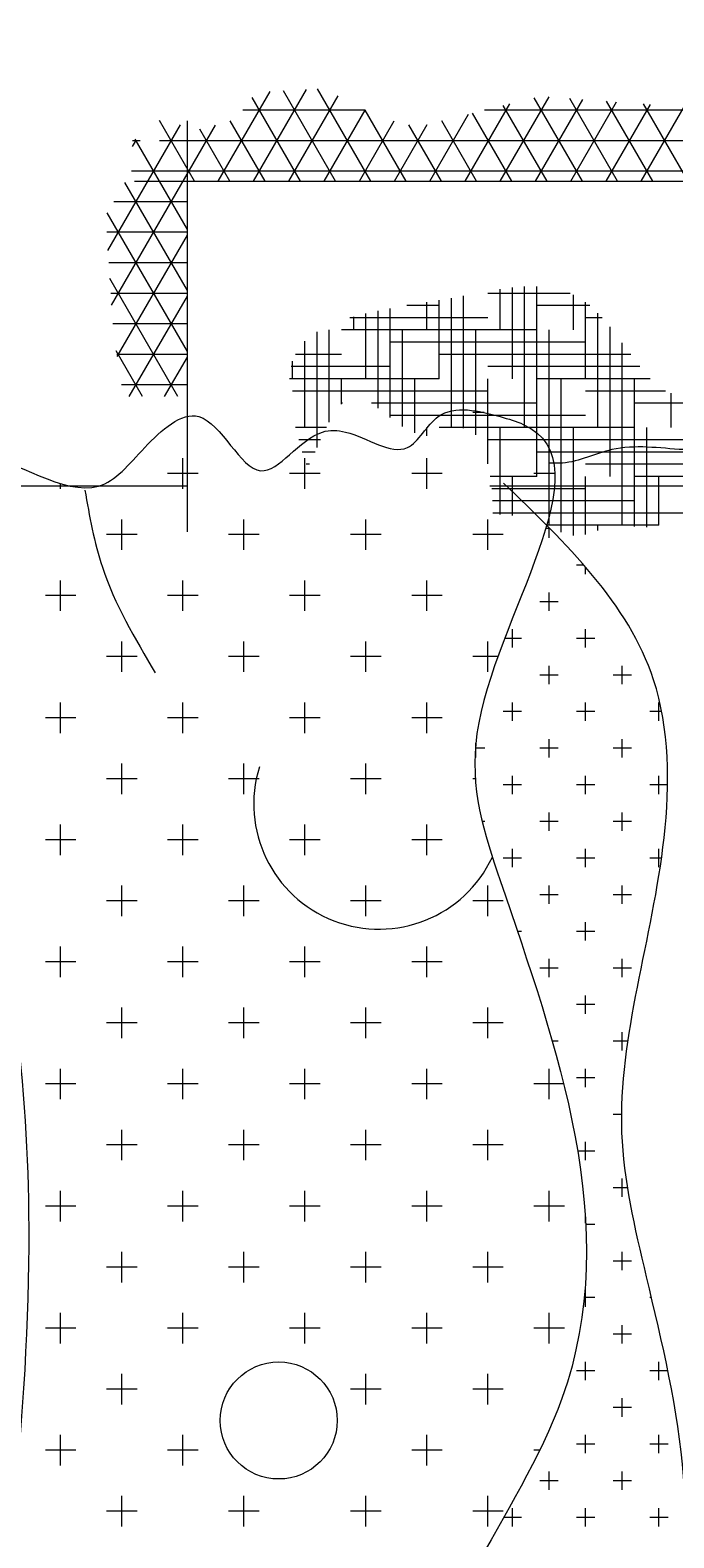
# Model space of a CAD drawing. Units: inches. Extents: x 3731 to 4318, y 1310 to 2388.
# Tile 5 of 57: x 3870 to 3897, y 1452 to 1515. Entities that reach past the tile are written whole.
import ezdxf

# ---------------------------------------------------------------- set-up
doc = ezdxf.new("R2010")
doc.units = ezdxf.units.IN
doc.layers.add('A-ANNO-DIMS', color=2, linetype='Continuous', lineweight=18)
doc.layers.add('A-FURN', color=8, linetype='Continuous', lineweight=13)
doc.styles.get("Standard").update_dxf_attribs({"font": 'arial.ttf'})
doc.dimstyles.get("Standard").update_dxf_attribs({"dimtxt": 0.18, "dimasz": 0.18, "dimexe": 0.18, "dimexo": 0.0625, "dimgap": 0.09, "dimtad": 0, "dimtih": 1, "dimtoh": 1, "dimdec": 4, "dimzin": 0, "dimdsep": 46, "dimtxsty": 'Standard', "dimcen": 0.09, "dimadec": 0, "dimazin": 0, "dimtfac": 1, "dimtdec": 4, "dimtofl": 0, "dimtmove": 0, "dimatfit": 3, "dimfxl": 1, "dimtolj": 1, "dimtzin": 0, "dimarcsym": 0})

# ---------------------------------------------------------------- blocks, each defined once
blk = doc.blocks.new('A$C200C7901')
for p, q in [((2, 1.6055), (2, 2.3334)), ((1.1379, 1.7195), (1.1379, 1.7508)), ((1.1222, 1.7352), (1.1535, 1.7352)), ((1.9972, 1.7352), (2.0027, 1.7352)), ((1.9972, 1.7352), (2.0027, 1.7352)), ((2, 1.6963), (2, 1.7248)), ((2, 1.6963), (2, 1.7248)), ((2.3121, 1.6596), (2.3121, 0.0201)), ((1.0129, 1.5945), (1.0129, 1.6258)), ((1.0129, 1.5945), (1.0129, 1.6258)), ((1.9533, 1.6055), (2.3741, 1.6055)), ((1.9533, 1.6055), (2.3741, 1.6055)), ((1.0754, 1.5625), (1.0754, 1.5633)), ((1.0754, 1.5625), (1.0754, 1.5633)), ((2, 0.2957), (2, 1.2957)), ((2.0224, 0.9977), (2.0224, 1.1977)), ((2.0224, 0.9977), (2.0224, 1.1977))]:
    blk.add_line(p, q)
at = {"linetype": 'ByBlock'}
for p, q in [((1.0129, 1.7195), (1.0129, 1.7508)), ((1.0129, 1.7195), (1.0129, 1.7508)), ((1.1379, 1.7195), (1.1379, 1.7508)), ((1.2629, 1.7195), (1.2629, 1.7508)), ((1.2629, 1.7195), (1.2629, 1.7508)), ((1.3879, 1.7195), (1.3879, 1.7508)), ((1.3879, 1.7195), (1.3879, 1.7508)), ((1.5129, 1.7195), (1.5129, 1.7508)), ((1.5129, 1.7195), (1.5129, 1.7508)), ((1.6379, 1.7195), (1.6379, 1.7508)), ((1.6379, 1.7195), (1.6379, 1.7508)), ((1.7629, 1.7195), (1.7629, 1.7508)), ((1.7629, 1.7195), (1.7629, 1.7508)), ((1.8879, 1.7195), (1.8879, 1.7508)), ((1.8879, 1.7195), (1.8879, 1.7508)), ((0.9972, 1.7352), (1.0285, 1.7352)), ((0.9972, 1.7352), (1.0285, 1.7352)), ((1.1222, 1.7352), (1.1535, 1.7352)), ((1.2472, 1.7352), (1.2785, 1.7352)), ((1.2472, 1.7352), (1.2785, 1.7352)), ((1.3722, 1.7352), (1.4035, 1.7352)), ((1.3722, 1.7352), (1.4035, 1.7352)), ((1.4972, 1.7352), (1.5285, 1.7352)), ((1.4972, 1.7352), (1.5285, 1.7352)), ((1.6222, 1.7352), (1.6535, 1.7352)), ((1.6222, 1.7352), (1.6535, 1.7352)), ((1.7472, 1.7352), (1.7785, 1.7352)), ((1.7472, 1.7352), (1.7785, 1.7352)), ((1.8722, 1.7352), (1.9035, 1.7352)), ((1.8722, 1.7352), (1.9035, 1.7352)), ((0.9504, 1.657), (0.9504, 1.6883)), ((0.9504, 1.657), (0.9504, 1.6883)), ((1.0754, 1.657), (1.0754, 1.6883)), ((1.0754, 1.657), (1.0754, 1.6883)), ((1.2004, 1.657), (1.2004, 1.6883)), ((1.2004, 1.657), (1.2004, 1.6883)), ((1.3254, 1.657), (1.3254, 1.6883)), ((1.3254, 1.657), (1.3254, 1.6883)), ((1.4504, 1.657), (1.4504, 1.6883)), ((1.4504, 1.657), (1.4504, 1.6883)), ((1.5754, 1.657), (1.5754, 1.6883)), ((1.5754, 1.657), (1.5754, 1.6883)), ((1.7004, 1.657), (1.7004, 1.6883)), ((1.7004, 1.657), (1.7004, 1.6883)), ((1.8254, 1.657), (1.8254, 1.6883)), ((1.8254, 1.657), (1.8254, 1.6883)), ((1.9504, 1.657), (1.9504, 1.6883)), ((1.9504, 1.657), (1.9504, 1.6883)), ((2.0919, 1.6152), (2.2125, 1.6848)), ((2.0919, 1.6152), (2.2125, 1.6848)), ((2.1377, 1.6055), (2.2798, 1.6876)), ((2.1377, 1.6055), (2.2798, 1.6876)), ((2.1854, 1.683), (2.3697, 1.5766)), ((2.1854, 1.683), (2.3697, 1.5766)), ((2.1974, 1.6055), (2.1974, 1.6838)), ((2.1974, 1.6055), (2.1974, 1.6838)), ((2.2287, 1.6055), (2.2287, 1.6859)), ((2.2287, 1.6055), (2.2287, 1.6859)), ((2.2414, 1.6868), (2.3699, 1.6126)), ((2.2414, 1.6868), (2.3699, 1.6126)), ((2.2599, 1.6055), (2.2599, 1.688)), ((2.2599, 1.6055), (2.2599, 1.688)), ((0.9347, 1.6727), (0.966, 1.6727)), ((0.9347, 1.6727), (0.966, 1.6727)), ((1.0597, 1.6727), (1.091, 1.6727)), ((1.0597, 1.6727), (1.091, 1.6727)), ((1.1847, 1.6727), (1.216, 1.6727)), ((1.1847, 1.6727), (1.216, 1.6727)), ((1.3097, 1.6727), (1.341, 1.6727)), ((1.3097, 1.6727), (1.341, 1.6727)), ((1.4347, 1.6727), (1.466, 1.6727)), ((1.4347, 1.6727), (1.466, 1.6727)), ((1.5597, 1.6727), (1.591, 1.6727)), ((1.5597, 1.6727), (1.591, 1.6727)), ((1.6847, 1.6727), (1.716, 1.6727)), ((1.6847, 1.6727), (1.716, 1.6727)), ((1.8097, 1.6727), (1.841, 1.6727)), ((1.8097, 1.6727), (1.841, 1.6727)), ((1.9347, 1.6727), (1.966, 1.6727)), ((1.9347, 1.6727), (1.966, 1.6727)), ((2.0919, 1.6513), (2.1386, 1.6782)), ((2.0919, 1.6513), (2.1386, 1.6782)), ((2.1037, 1.6055), (2.1037, 1.673)), ((2.1037, 1.6055), (2.1037, 1.673)), ((2.1327, 1.6773), (2.2571, 1.6055)), ((2.1327, 1.6773), (2.2571, 1.6055)), ((2.1349, 1.6055), (2.1349, 1.6777)), ((2.1349, 1.6055), (2.1349, 1.6777)), ((2.1662, 1.6055), (2.1662, 1.6817)), ((2.1662, 1.6055), (2.1662, 1.6817)), ((2.2002, 1.6055), (2.3109, 1.6694)), ((2.2002, 1.6055), (2.3109, 1.6694)), ((2.2912, 1.6055), (2.2912, 1.6809)), ((2.2912, 1.6055), (2.2912, 1.6809)), ((2.0919, 1.6649), (2.1946, 1.6055)), ((2.0919, 1.6649), (2.1946, 1.6055)), ((2.2627, 1.6055), (2.3551, 1.6589)), ((2.2627, 1.6055), (2.3551, 1.6589)), ((2.3224, 0.0468), (2.3224, 1.6627)), ((2.3224, 0.0468), (2.3224, 1.6627)), ((2.3476, 1.6616), (2.3547, 1.6575)), ((2.3476, 1.6616), (2.3547, 1.6575)), ((2.3537, 1.6539), (2.3537, 1.6616)), ((2.3537, 1.6539), (2.3537, 1.6616)), ((1.1379, 1.5945), (1.1379, 1.6258)), ((1.1379, 1.5945), (1.1379, 1.6258)), ((1.2629, 1.5945), (1.2629, 1.6258)), ((1.2629, 1.5945), (1.2629, 1.6258)), ((1.3879, 1.5945), (1.3879, 1.6258)), ((1.3879, 1.5945), (1.3879, 1.6258)), ((1.5129, 1.5945), (1.5129, 1.6258)), ((1.5129, 1.5945), (1.5129, 1.6258)), ((1.6379, 1.5945), (1.6379, 1.6258)), ((1.6379, 1.5945), (1.6379, 1.6258)), ((1.7629, 1.5945), (1.7629, 1.6258)), ((1.7629, 1.5945), (1.7629, 1.6258)), ((1.8879, 1.5945), (1.8879, 1.6258)), ((1.8879, 1.5945), (1.8879, 1.6258)), ((2.0129, 1.5945), (2.0129, 1.6258)), ((2.0129, 1.5945), (2.0129, 1.6258)), ((2.0919, 1.6288), (2.1321, 1.6055)), ((2.0919, 1.6288), (2.1321, 1.6055)), ((2.3121, 1.598), (2.3745, 1.634)), ((2.3121, 1.598), (2.3745, 1.634)), ((2.3537, 0.0056), (2.3537, 1.634)), ((2.3537, 0.0056), (2.3537, 1.634)), ((0.9972, 1.6102), (1.0285, 1.6102)), ((0.9972, 1.6102), (1.0285, 1.6102)), ((1.1222, 1.6102), (1.1535, 1.6102)), ((1.1222, 1.6102), (1.1535, 1.6102)), ((1.2472, 1.6102), (1.2785, 1.6102)), ((1.2472, 1.6102), (1.2785, 1.6102)), ((1.3722, 1.6102), (1.4035, 1.6102)), ((1.3722, 1.6102), (1.4035, 1.6102)), ((1.4972, 1.6102), (1.5285, 1.6102)), ((1.4972, 1.6102), (1.5285, 1.6102)), ((1.6222, 1.6102), (1.6535, 1.6102)), ((1.6222, 1.6102), (1.6535, 1.6102)), ((1.7472, 1.6102), (1.7785, 1.6102)), ((1.7472, 1.6102), (1.7785, 1.6102)), ((1.8722, 1.6102), (1.9035, 1.6102)), ((1.8722, 1.6102), (1.9035, 1.6102)), ((1.9972, 1.6102), (2.0285, 1.6102)), ((1.9972, 1.6102), (2.0285, 1.6102)), ((2.3121, 1.5619), (2.3654, 1.5926)), ((2.3121, 1.5619), (2.3654, 1.5926)), ((0.9504, 1.532), (0.9504, 1.5633)), ((0.9504, 1.532), (0.9504, 1.5633)), ((1.2004, 1.532), (1.2004, 1.5633)), ((1.2004, 1.532), (1.2004, 1.5633)), ((1.3254, 1.532), (1.3254, 1.5633)), ((1.3254, 1.532), (1.3254, 1.5633)), ((1.4504, 1.532), (1.4504, 1.5633)), ((1.4504, 1.532), (1.4504, 1.5633)), ((1.5754, 1.532), (1.5754, 1.5633)), ((1.5754, 1.532), (1.5754, 1.5633)), ((1.7004, 1.532), (1.7004, 1.5633)), ((1.7004, 1.532), (1.7004, 1.5633)), ((1.8254, 1.532), (1.8254, 1.5633)), ((1.8254, 1.532), (1.8254, 1.5633)), ((1.9504, 1.532), (1.9504, 1.5633)), ((1.9504, 1.532), (1.9504, 1.5633)), ((2.3121, 1.5738), (2.404, 1.5208)), ((2.3121, 1.5738), (2.404, 1.5208)), ((2.3121, 1.5258), (2.3739, 1.5615)), ((2.3121, 1.5258), (2.3739, 1.5615)), ((0.9347, 1.5477), (0.966, 1.5477)), ((0.9347, 1.5477), (0.966, 1.5477)), ((1.1847, 1.5477), (1.216, 1.5477)), ((1.1847, 1.5477), (1.216, 1.5477)), ((1.3097, 1.5477), (1.341, 1.5477)), ((1.3097, 1.5477), (1.341, 1.5477)), ((1.4347, 1.5477), (1.466, 1.5477)), ((1.4347, 1.5477), (1.466, 1.5477)), ((1.5597, 1.5477), (1.591, 1.5477)), ((1.5597, 1.5477), (1.591, 1.5477)), ((1.6847, 1.5477), (1.716, 1.5477)), ((1.6847, 1.5477), (1.716, 1.5477)), ((1.8097, 1.5477), (1.841, 1.5477)), ((1.8097, 1.5477), (1.841, 1.5477)), ((1.9347, 1.5477), (1.966, 1.5477)), ((1.9347, 1.5477), (1.966, 1.5477)), ((2.3849, 1.4236), (2.3849, 1.5486)), ((2.3849, 1.4236), (2.3849, 1.5486)), ((2.3121, 1.4897), (2.3979, 1.5393)), ((2.3121, 1.4897), (2.3979, 1.5393)), ((2.3121, 1.5377), (2.406, 1.4835)), ((2.3121, 1.5377), (2.406, 1.4835)), ((1.1379, 1.4695), (1.1379, 1.5008)), ((1.1379, 1.4695), (1.1379, 1.5008)), ((1.2629, 1.4695), (1.2629, 1.5008)), ((1.2629, 1.4695), (1.2629, 1.5008)), ((1.3879, 1.4695), (1.3879, 1.5008)), ((1.3879, 1.4695), (1.3879, 1.5008)), ((1.5129, 1.4695), (1.5129, 1.5008)), ((1.5129, 1.4695), (1.5129, 1.5008)), ((1.6379, 1.4695), (1.6379, 1.5008)), ((1.6379, 1.4695), (1.6379, 1.5008)), ((1.7629, 1.4695), (1.7629, 1.5008)), ((1.7629, 1.4695), (1.7629, 1.5008)), ((1.8879, 1.4695), (1.8879, 1.5008)), ((1.8879, 1.4695), (1.8879, 1.5008)), ((2.0129, 1.4695), (2.0129, 1.5008)), ((2.0129, 1.4695), (2.0129, 1.5008)), ((2.0974, 1.2977), (2.0974, 1.4977)), ((2.0974, 1.2977), (2.0974, 1.4977)), ((2.1099, 1.3477), (2.1099, 1.5009)), ((2.1099, 1.3477), (2.1099, 1.5009)), ((2.1099, 1.4977), (2.1279, 1.4977)), ((2.1099, 1.4977), (2.1279, 1.4977)), ((2.1224, 1.3977), (2.1224, 1.4992)), ((2.1224, 1.3977), (2.1224, 1.4992)), ((2.3121, 1.4537), (2.4047, 1.5071)), ((2.3121, 1.4537), (2.4047, 1.5071)), ((2.3121, 1.5016), (2.3997, 1.4511)), ((2.3121, 1.5016), (2.3997, 1.4511)), ((1.1222, 1.4852), (1.1535, 1.4852)), ((1.1222, 1.4852), (1.1535, 1.4852)), ((1.2472, 1.4852), (1.2785, 1.4852)), ((1.2472, 1.4852), (1.2785, 1.4852)), ((1.3722, 1.4852), (1.4035, 1.4852)), ((1.3722, 1.4852), (1.4035, 1.4852)), ((1.4972, 1.4852), (1.5285, 1.4852)), ((1.4972, 1.4852), (1.5285, 1.4852)), ((1.6222, 1.4852), (1.6535, 1.4852)), ((1.6222, 1.4852), (1.6535, 1.4852)), ((1.7472, 1.4852), (1.7785, 1.4852)), ((1.7472, 1.4852), (1.7785, 1.4852)), ((1.8722, 1.4852), (1.9035, 1.4852)), ((1.8722, 1.4852), (1.9035, 1.4852)), ((1.9972, 1.4852), (2.0285, 1.4852)), ((1.9972, 1.4852), (2.0285, 1.4852)), ((2.0224, 1.4805), (2.0224, 1.4839)), ((2.0224, 1.4805), (2.0224, 1.4839)), ((2.0349, 1.4748), (2.0349, 1.4879)), ((2.0349, 1.4748), (2.0349, 1.4879)), ((2.0474, 1.4691), (2.0474, 1.4915)), ((2.0474, 1.4691), (2.0474, 1.4915)), ((2.0599, 1.4631), (2.0599, 1.4948)), ((2.0599, 1.4631), (2.0599, 1.4948)), ((2.0599, 1.4852), (2.1484, 1.4852)), ((2.0599, 1.4852), (2.1484, 1.4852)), ((2.1349, 1.4477), (2.1349, 1.4949)), ((2.1349, 1.4477), (2.1349, 1.4949)), ((2.0397, 1.4727), (2.1581, 1.4727)), ((2.0397, 1.4727), (2.1581, 1.4727)), ((2.3121, 1.4176), (2.4067, 1.4721)), ((2.3121, 1.4176), (2.4067, 1.4721)), ((2.0656, 1.4602), (2.1599, 1.4602)), ((2.0656, 1.4602), (2.1599, 1.4602)), ((2.3121, 1.4655), (2.3849, 1.4235)), ((2.3121, 1.4655), (2.3849, 1.4235)), ((0.9504, 1.407), (0.9504, 1.4383)), ((0.9504, 1.407), (0.9504, 1.4383)), ((1.0754, 1.407), (1.0754, 1.4383)), ((1.0754, 1.407), (1.0754, 1.4383)), ((1.2004, 1.407), (1.2004, 1.4383)), ((1.2004, 1.407), (1.2004, 1.4383)), ((1.3254, 1.407), (1.3254, 1.4383)), ((1.3254, 1.407), (1.3254, 1.4383)), ((1.4504, 1.407), (1.4504, 1.4383)), ((1.4504, 1.407), (1.4504, 1.4383)), ((1.5754, 1.407), (1.5754, 1.4383)), ((1.5754, 1.407), (1.5754, 1.4383)), ((1.7004, 1.407), (1.7004, 1.4383)), ((1.7004, 1.407), (1.7004, 1.4383)), ((1.8254, 1.407), (1.8254, 1.4383)), ((1.8254, 1.407), (1.8254, 1.4383)), ((1.9504, 1.407), (1.9504, 1.4383)), ((1.9504, 1.407), (1.9504, 1.4383)), ((2.084, 1.4477), (2.1099, 1.4477)), ((2.084, 1.4477), (2.1099, 1.4477)), ((2.0849, 1.4468), (2.0849, 1.4477)), ((2.0849, 1.4468), (2.0849, 1.4477)), ((2.1599, 1.2477), (2.1599, 1.4477)), ((2.1599, 1.2477), (2.1599, 1.4477)), ((2.1724, 1.2977), (2.1724, 1.439)), ((2.1724, 1.2977), (2.1724, 1.439)), ((0.9347, 1.4227), (0.966, 1.4227)), ((0.9347, 1.4227), (0.966, 1.4227)), ((1.0597, 1.4227), (1.091, 1.4227)), ((1.0597, 1.4227), (1.091, 1.4227)), ((1.1847, 1.4227), (1.216, 1.4227)), ((1.1847, 1.4227), (1.216, 1.4227)), ((1.3097, 1.4227), (1.341, 1.4227)), ((1.3097, 1.4227), (1.341, 1.4227)), ((1.4347, 1.4227), (1.466, 1.4227)), ((1.4347, 1.4227), (1.466, 1.4227)), ((1.5597, 1.4227), (1.591, 1.4227)), ((1.5597, 1.4227), (1.591, 1.4227)), ((1.6847, 1.4227), (1.716, 1.4227)), ((1.6847, 1.4227), (1.716, 1.4227)), ((1.8097, 1.4227), (1.841, 1.4227)), ((1.8097, 1.4227), (1.841, 1.4227)), ((1.9347, 1.4227), (1.966, 1.4227)), ((1.9347, 1.4227), (1.966, 1.4227)), ((2.1099, 1.4227), (2.1767, 1.4227)), ((2.1099, 1.4227), (2.1767, 1.4227)), ((2.1599, 1.4352), (2.1735, 1.4352)), ((2.1599, 1.4352), (2.1735, 1.4352)), ((2.3121, 1.4294), (2.3741, 1.3937)), ((2.3121, 1.4294), (2.3741, 1.3937)), ((2.3121, 1.3815), (2.3848, 1.4235)), ((2.3121, 1.3815), (2.3848, 1.4235)), ((2.08, 1.4102), (2.1795, 1.4102)), ((2.08, 1.4102), (2.1795, 1.4102)), ((2.0849, 1.2477), (2.0849, 1.4171)), ((2.0849, 1.2477), (2.0849, 1.4171)), ((2.0703, 1.3977), (2.1819, 1.3977)), ((2.0703, 1.3977), (2.1819, 1.3977)), ((2.0724, 1.1977), (2.0724, 1.3977)), ((2.0724, 1.1977), (2.0724, 1.3977)), ((2.1474, 1.1977), (2.1474, 1.3977)), ((2.1474, 1.1977), (2.1474, 1.3977)), ((2.3121, 1.3934), (2.3703, 1.3598)), ((2.3121, 1.3934), (2.3703, 1.3598)), ((1.0129, 1.3445), (1.0129, 1.3758)), ((1.0129, 1.3445), (1.0129, 1.3758)), ((1.1379, 1.3445), (1.1379, 1.3758)), ((1.1379, 1.3445), (1.1379, 1.3758)), ((1.2629, 1.3445), (1.2629, 1.3758)), ((1.2629, 1.3445), (1.2629, 1.3758)), ((1.3879, 1.3445), (1.3879, 1.3758)), ((1.3879, 1.3445), (1.3879, 1.3758)), ((1.5129, 1.3445), (1.5129, 1.3758)), ((1.5129, 1.3445), (1.5129, 1.3758)), ((1.6379, 1.3445), (1.6379, 1.3758)), ((1.6379, 1.3445), (1.6379, 1.3758)), ((1.7629, 1.3445), (1.7629, 1.3758)), ((1.7629, 1.3445), (1.7629, 1.3758)), ((1.8879, 1.3445), (1.8879, 1.3758)), ((1.8879, 1.3445), (1.8879, 1.3758)), ((2.0129, 1.3445), (2.0129, 1.3758)), ((2.0129, 1.3445), (2.0129, 1.3758)), ((2.0612, 1.3852), (2.1599, 1.3852)), ((2.0612, 1.3852), (2.1599, 1.3852)), ((2.1849, 1.3477), (2.1849, 1.3808)), ((2.1849, 1.3477), (2.1849, 1.3808)), ((2.3121, 1.3454), (2.37, 1.3788)), ((2.3121, 1.3454), (2.37, 1.3788)), ((0.9972, 1.3602), (1.0285, 1.3602)), ((0.9972, 1.3602), (1.0285, 1.3602)), ((1.1222, 1.3602), (1.1535, 1.3602)), ((1.1222, 1.3602), (1.1535, 1.3602)), ((1.2472, 1.3602), (1.2785, 1.3602)), ((1.2472, 1.3602), (1.2785, 1.3602)), ((1.3722, 1.3602), (1.4035, 1.3602)), ((1.3722, 1.3602), (1.4035, 1.3602)), ((1.4972, 1.3602), (1.5285, 1.3602)), ((1.4972, 1.3602), (1.5285, 1.3602)), ((1.6222, 1.3602), (1.6535, 1.3602)), ((1.6222, 1.3602), (1.6535, 1.3602)), ((1.7472, 1.3602), (1.7785, 1.3602)), ((1.7472, 1.3602), (1.7785, 1.3602)), ((1.8722, 1.3602), (1.9035, 1.3602)), ((1.8722, 1.3602), (1.9035, 1.3602)), ((1.9972, 1.3602), (2.0285, 1.3602)), ((1.9972, 1.3602), (2.0285, 1.3602)), ((2.0515, 1.3602), (2.0599, 1.3602)), ((2.0515, 1.3602), (2.0599, 1.3602)), ((2.0545, 1.3727), (2.1099, 1.3727)), ((2.0545, 1.3727), (2.1099, 1.3727)), ((2.1599, 1.3602), (2.1883, 1.3602)), ((2.1599, 1.3602), (2.1883, 1.3602)), ((2.0599, 1.1477), (2.0599, 1.3477)), ((2.0599, 1.1477), (2.0599, 1.3477)), ((2.1099, 1.3477), (2.1904, 1.3477)), ((2.1099, 1.3477), (2.1904, 1.3477)), ((2.1349, 1.1515), (2.1349, 1.3477)), ((2.1349, 1.1515), (2.1349, 1.3477)), ((2.3121, 1.3573), (2.3808, 1.3176)), ((2.3121, 1.3573), (2.3808, 1.3176)), ((2.3121, 1.3093), (2.374, 1.345)), ((2.3121, 1.3093), (2.374, 1.345)), ((2.0599, 1.3352), (2.1926, 1.3352)), ((2.0599, 1.3352), (2.1926, 1.3352)), ((0.9504, 1.282), (0.9504, 1.3133)), ((0.9504, 1.282), (0.9504, 1.3133)), ((1.0754, 1.282), (1.0754, 1.3133)), ((1.0754, 1.282), (1.0754, 1.3133)), ((1.2004, 1.282), (1.2004, 1.3133)), ((1.2004, 1.282), (1.2004, 1.3133)), ((1.3254, 1.282), (1.3254, 1.3133)), ((1.3254, 1.282), (1.3254, 1.3133)), ((1.4504, 1.282), (1.4504, 1.3133)), ((1.4504, 1.282), (1.4504, 1.3133)), ((1.5754, 1.282), (1.5754, 1.3133)), ((1.5754, 1.282), (1.5754, 1.3133)), ((1.7004, 1.3106), (1.7004, 1.3133)), ((1.7004, 1.3106), (1.7004, 1.3133)), ((1.8254, 1.2876), (1.8254, 1.3133)), ((1.8254, 1.2876), (1.8254, 1.3133)), ((1.9504, 1.282), (1.9504, 1.3133)), ((1.9504, 1.282), (1.9504, 1.3133)), ((2.0594, 1.3227), (2.195, 1.3227)), ((2.0594, 1.3227), (2.195, 1.3227)), ((2.0754, 1.3017), (2.0754, 1.3133)), ((2.0754, 1.3017), (2.0754, 1.3133)), ((2.3121, 1.3212), (2.3914, 1.2754)), ((2.3121, 1.3212), (2.3914, 1.2754)), ((2.3121, 1.2732), (2.3819, 1.3135)), ((2.3121, 1.2732), (2.3819, 1.3135)), ((0.9347, 1.2977), (0.966, 1.2977)), ((0.9347, 1.2977), (0.966, 1.2977)), ((1.0597, 1.2977), (1.091, 1.2977)), ((1.0597, 1.2977), (1.091, 1.2977)), ((1.1847, 1.2977), (1.216, 1.2977)), ((1.1847, 1.2977), (1.216, 1.2977)), ((1.3097, 1.2977), (1.341, 1.2977)), ((1.3097, 1.2977), (1.341, 1.2977)), ((1.4347, 1.2977), (1.466, 1.2977)), ((1.4347, 1.2977), (1.466, 1.2977)), ((1.5597, 1.2977), (1.591, 1.2977)), ((1.5597, 1.2977), (1.591, 1.2977)), ((1.6566, 1.3008), (1.6566, 1.3036)), ((1.6566, 1.3008), (1.6566, 1.3036)), ((1.7222, 1.3102), (1.7369, 1.3102)), ((1.7222, 1.3102), (1.7369, 1.3102)), ((1.7316, 1.3008), (1.7316, 1.3106)), ((1.7316, 1.3008), (1.7316, 1.3106)), ((1.8097, 1.2977), (1.841, 1.2977)), ((1.8097, 1.2977), (1.841, 1.2977)), ((1.9347, 1.2977), (1.966, 1.2977)), ((1.9347, 1.2977), (1.966, 1.2977)), ((2.023, 1.2977), (2.1099, 1.2977)), ((2.023, 1.2977), (2.1099, 1.2977)), ((2.0474, 1.0977), (2.0474, 1.2977)), ((2.0474, 1.0977), (2.0474, 1.2977)), ((2.0524, 1.3102), (2.1599, 1.3102)), ((2.0524, 1.3102), (2.1599, 1.3102)), ((2.0597, 1.2977), (2.0744, 1.2977)), ((2.0597, 1.2977), (2.0744, 1.2977)), ((2.1224, 1.1421), (2.1224, 1.2977)), ((2.1224, 1.1421), (2.1224, 1.2977)), ((2.1974, 1.2135), (2.1974, 1.2977)), ((2.1974, 1.2135), (2.1974, 1.2977)), ((2.3849, 1.0607), (2.3849, 1.3013)), ((2.3849, 1.0607), (2.3849, 1.3013)), ((0.9441, 1.2633), (0.9441, 1.2816)), ((0.9441, 1.2633), (0.9441, 1.2816)), ((1.6191, 1.2633), (1.6191, 1.282)), ((1.6191, 1.2633), (1.6191, 1.282)), ((1.6941, 1.2633), (1.6941, 1.282)), ((1.6941, 1.2633), (1.6941, 1.282)), ((1.7691, 1.2633), (1.7691, 1.282)), ((1.7691, 1.2633), (1.7691, 1.282)), ((1.9711, 1.2852), (2.0599, 1.2852)), ((1.9711, 1.2852), (2.0599, 1.2852)), ((1.9724, 1.0977), (1.9724, 1.2927)), ((1.9724, 1.0977), (1.9724, 1.2927)), ((1.9849, 1.1477), (1.9849, 1.293)), ((1.9849, 1.1477), (1.9849, 1.293)), ((1.9974, 1.1977), (1.9974, 1.2939)), ((1.9974, 1.1977), (1.9974, 1.2939)), ((2.0099, 1.2477), (2.0099, 1.2953)), ((2.0099, 1.2477), (2.0099, 1.2953)), ((2.1599, 1.2852), (2.2018, 1.2852)), ((2.1599, 1.2852), (2.2018, 1.2852)), ((2.3121, 1.2851), (2.3985, 1.2352)), ((2.3121, 1.2851), (2.3985, 1.2352)), ((2.3121, 1.2371), (2.3898, 1.282)), ((2.3121, 1.2371), (2.3898, 1.282)), ((0.9347, 1.2727), (0.9535, 1.2727)), ((0.9347, 1.2727), (0.9535, 1.2727)), ((1.5441, 1.2633), (1.5441, 1.2675)), ((1.5441, 1.2633), (1.5441, 1.2675)), ((1.6097, 1.2727), (1.6285, 1.2727)), ((1.6097, 1.2727), (1.6285, 1.2727)), ((1.6847, 1.2727), (1.7035, 1.2727)), ((1.6847, 1.2727), (1.7035, 1.2727)), ((1.7597, 1.2727), (1.7785, 1.2727)), ((1.7597, 1.2727), (1.7785, 1.2727)), ((1.8347, 1.2727), (1.8535, 1.2727)), ((1.8347, 1.2727), (1.8535, 1.2727)), ((1.8441, 1.2633), (1.8441, 1.2806)), ((1.8441, 1.2633), (1.8441, 1.2806)), ((1.97, 1.2727), (2.0099, 1.2727)), ((1.97, 1.2727), (2.0099, 1.2727)), ((2.1099, 1.2727), (2.2034, 1.2727)), ((2.1099, 1.2727), (2.2034, 1.2727)), ((1.0129, 1.2448), (1.0129, 1.2508)), ((1.0129, 1.2448), (1.0129, 1.2508)), ((1.1379, 1.2195), (1.1379, 1.2508)), ((1.1379, 1.2195), (1.1379, 1.2508)), ((1.2629, 1.2195), (1.2629, 1.2508)), ((1.2629, 1.2195), (1.2629, 1.2508)), ((1.3879, 1.2202), (1.3879, 1.2508)), ((1.3879, 1.2202), (1.3879, 1.2508)), ((2.0129, 1.2293), (2.0129, 1.2508)), ((2.0129, 1.2293), (2.0129, 1.2508)), ((2.0599, 1.2602), (2.2044, 1.2602)), ((2.0599, 1.2602), (2.2044, 1.2602)), ((2.3121, 1.2011), (2.3976, 1.2504)), ((2.3121, 1.2011), (2.3976, 1.2504)), ((0.9722, 1.2352), (0.991, 1.2352)), ((0.9722, 1.2352), (0.991, 1.2352)), ((0.9816, 1.2258), (0.9816, 1.2445)), ((0.9816, 1.2258), (0.9816, 1.2445)), ((1.1222, 1.2352), (1.1535, 1.2352)), ((1.1222, 1.2352), (1.1535, 1.2352)), ((1.2472, 1.2352), (1.2785, 1.2352)), ((1.2472, 1.2352), (1.2785, 1.2352)), ((1.3722, 1.2352), (1.4035, 1.2352)), ((1.3722, 1.2352), (1.4035, 1.2352)), ((1.4972, 1.2352), (1.516, 1.2352)), ((1.4972, 1.2352), (1.516, 1.2352)), ((1.5066, 1.2258), (1.5066, 1.2445)), ((1.5066, 1.2258), (1.5066, 1.2445)), ((1.5722, 1.2352), (1.591, 1.2352)), ((1.5722, 1.2352), (1.591, 1.2352)), ((1.5816, 1.2258), (1.5816, 1.2445)), ((1.5816, 1.2258), (1.5816, 1.2445)), ((1.6472, 1.2352), (1.666, 1.2352)), ((1.6472, 1.2352), (1.666, 1.2352)), ((1.6566, 1.2258), (1.6566, 1.2445)), ((1.6566, 1.2258), (1.6566, 1.2445)), ((1.7222, 1.2352), (1.741, 1.2352)), ((1.7222, 1.2352), (1.741, 1.2352)), ((1.7316, 1.2258), (1.7316, 1.2445)), ((1.7316, 1.2258), (1.7316, 1.2445)), ((1.7972, 1.2352), (1.816, 1.2352)), ((1.7972, 1.2352), (1.816, 1.2352)), ((1.8066, 1.2258), (1.8066, 1.2445)), ((1.8066, 1.2258), (1.8066, 1.2445)), ((1.8722, 1.2352), (1.891, 1.2352)), ((1.8722, 1.2352), (1.891, 1.2352)), ((1.8816, 1.2258), (1.8816, 1.2445)), ((1.8816, 1.2258), (1.8816, 1.2445)), ((1.9472, 1.2352), (1.9574, 1.2352)), ((1.9472, 1.2352), (1.9574, 1.2352)), ((1.9566, 1.2344), (1.9566, 1.2385)), ((1.9566, 1.2344), (1.9566, 1.2385)), ((1.9599, 1.1228), (1.9599, 1.2373)), ((1.9599, 1.1228), (1.9599, 1.2373)), ((1.9599, 1.2352), (2.1599, 1.2352)), ((1.9599, 1.2352), (2.1599, 1.2352)), ((2, 1.2352), (2.0285, 1.2352)), ((2, 1.2352), (2.0285, 1.2352)), ((2.0099, 1.2477), (2.2045, 1.2477)), ((2.0099, 1.2477), (2.2045, 1.2477)), ((2.0349, 1.0477), (2.0349, 1.2477)), ((2.0349, 1.0477), (2.0349, 1.2477)), ((2.1099, 1.1315), (2.1099, 1.2477)), ((2.1099, 1.1315), (2.1099, 1.2477)), ((2.1849, 1.1935), (2.1849, 1.2477)), ((2.1849, 1.1935), (2.1849, 1.2477)), ((2.3121, 1.249), (2.396, 1.2006)), ((2.3121, 1.249), (2.396, 1.2006)), ((1.4316, 1.2258), (1.4316, 1.2318)), ((1.4316, 1.2258), (1.4316, 1.2318)), ((1.953, 1.2227), (2.1099, 1.2227)), ((1.953, 1.2227), (2.1099, 1.2227)), ((0.9441, 1.1883), (0.9441, 1.207)), ((0.9441, 1.1883), (0.9441, 1.207)), ((1.0191, 1.1883), (1.0191, 1.207)), ((1.0191, 1.1883), (1.0191, 1.207)), ((1.0941, 1.1883), (1.0941, 1.207)), ((1.0941, 1.1883), (1.0941, 1.207)), ((1.3191, 1.1883), (1.3191, 1.2059)), ((1.3191, 1.1883), (1.3191, 1.2059)), ((1.3941, 1.1883), (1.3941, 1.207)), ((1.3941, 1.1883), (1.3941, 1.207)), ((1.4691, 1.1883), (1.4691, 1.207)), ((1.4691, 1.1883), (1.4691, 1.207)), ((1.5441, 1.1883), (1.5441, 1.207)), ((1.5441, 1.1883), (1.5441, 1.207)), ((1.6191, 1.1883), (1.6191, 1.207)), ((1.6191, 1.1883), (1.6191, 1.207)), ((1.6941, 1.1883), (1.6941, 1.207)), ((1.6941, 1.1883), (1.6941, 1.207)), ((1.7691, 1.1883), (1.7691, 1.207)), ((1.7691, 1.1883), (1.7691, 1.207)), ((1.8441, 1.1883), (1.8441, 1.207)), ((1.8441, 1.1883), (1.8441, 1.207)), ((1.9191, 1.1995), (1.9191, 1.207)), ((1.9191, 1.1995), (1.9191, 1.207)), ((1.9495, 1.2102), (2.0599, 1.2102)), ((1.9495, 1.2102), (2.0599, 1.2102)), ((2.1599, 1.2102), (2.1959, 1.2102)), ((2.1599, 1.2102), (2.1959, 1.2102)), ((2.3121, 1.165), (2.397, 1.214)), ((2.3121, 1.165), (2.397, 1.214)), ((2.3121, 1.2129), (2.3935, 1.166)), ((2.3121, 1.2129), (2.3935, 1.166)), ((0.9347, 1.1977), (0.9535, 1.1977)), ((0.9347, 1.1977), (0.9535, 1.1977)), ((1.0097, 1.1977), (1.0285, 1.1977)), ((1.0097, 1.1977), (1.0285, 1.1977)), ((1.0847, 1.1977), (1.1035, 1.1977)), ((1.0847, 1.1977), (1.1035, 1.1977)), ((1.1597, 1.1977), (1.1785, 1.1977)), ((1.1597, 1.1977), (1.1785, 1.1977)), ((1.1691, 1.1883), (1.1691, 1.1991)), ((1.1691, 1.1883), (1.1691, 1.1991)), ((1.2441, 1.1883), (1.2441, 1.1976)), ((1.2441, 1.1883), (1.2441, 1.1976)), ((1.2452, 1.1977), (1.2535, 1.1977)), ((1.2452, 1.1977), (1.2535, 1.1977)), ((1.3097, 1.1977), (1.3285, 1.1977)), ((1.3097, 1.1977), (1.3285, 1.1977)), ((1.3847, 1.1977), (1.4035, 1.1977)), ((1.3847, 1.1977), (1.4035, 1.1977)), ((1.4597, 1.1977), (1.4785, 1.1977)), ((1.4597, 1.1977), (1.4785, 1.1977)), ((1.5347, 1.1977), (1.5535, 1.1977)), ((1.5347, 1.1977), (1.5535, 1.1977)), ((1.6097, 1.1977), (1.6285, 1.1977)), ((1.6097, 1.1977), (1.6285, 1.1977)), ((1.6847, 1.1977), (1.7035, 1.1977)), ((1.6847, 1.1977), (1.7035, 1.1977)), ((1.7597, 1.1977), (1.7785, 1.1977)), ((1.7597, 1.1977), (1.7785, 1.1977)), ((1.8347, 1.1977), (1.8535, 1.1977)), ((1.8347, 1.1977), (1.8535, 1.1977)), ((1.9097, 1.1977), (1.917, 1.1977)), ((1.9097, 1.1977), (1.917, 1.1977)), ((1.9506, 1.1977), (2.0099, 1.1977)), ((1.9506, 1.1977), (2.0099, 1.1977)), ((2.0974, 1.1161), (2.0974, 1.1977)), ((2.0974, 1.1161), (2.0974, 1.1977)), ((2.1099, 1.1977), (2.1882, 1.1977)), ((2.1099, 1.1977), (2.1882, 1.1977)), ((2.1724, 1.1807), (2.1724, 1.1977)), ((2.1724, 1.1807), (2.1724, 1.1977)), ((1.9545, 1.1852), (1.9599, 1.1852)), ((1.9545, 1.1852), (1.9599, 1.1852)), ((2.0599, 1.1852), (2.1772, 1.1852)), ((2.0599, 1.1852), (2.1772, 1.1852)), ((2.3121, 1.1768), (2.3909, 1.1314)), ((2.3121, 1.1768), (2.3909, 1.1314)), ((2.3121, 1.1289), (2.3942, 1.1763)), ((2.3121, 1.1289), (2.3942, 1.1763)), ((0.9722, 1.1602), (0.991, 1.1602)), ((0.9722, 1.1602), (0.991, 1.1602)), ((0.9816, 1.1508), (0.9816, 1.1695)), ((0.9816, 1.1508), (0.9816, 1.1695)), ((1.0472, 1.1602), (1.066, 1.1602)), ((1.0472, 1.1602), (1.066, 1.1602)), ((1.0566, 1.1508), (1.0566, 1.1695)), ((1.0566, 1.1508), (1.0566, 1.1695)), ((1.1222, 1.1602), (1.141, 1.1602)), ((1.1222, 1.1602), (1.141, 1.1602)), ((1.1316, 1.1508), (1.1316, 1.1695)), ((1.1316, 1.1508), (1.1316, 1.1695)), ((1.1972, 1.1602), (1.216, 1.1602)), ((1.1972, 1.1602), (1.216, 1.1602)), ((1.2066, 1.1508), (1.2066, 1.1695)), ((1.2066, 1.1508), (1.2066, 1.1695)), ((1.2722, 1.1602), (1.291, 1.1602)), ((1.2722, 1.1602), (1.291, 1.1602)), ((1.2816, 1.1547), (1.2816, 1.1695)), ((1.2816, 1.1547), (1.2816, 1.1695)), ((1.3566, 1.1608), (1.3566, 1.1695)), ((1.3566, 1.1608), (1.3566, 1.1695)), ((1.4222, 1.1602), (1.441, 1.1602)), ((1.4222, 1.1602), (1.441, 1.1602)), ((1.4316, 1.1544), (1.4316, 1.1695)), ((1.4316, 1.1544), (1.4316, 1.1695)), ((1.4972, 1.1602), (1.516, 1.1602)), ((1.4972, 1.1602), (1.516, 1.1602)), ((1.5066, 1.1508), (1.5066, 1.1695)), ((1.5066, 1.1508), (1.5066, 1.1695)), ((1.5722, 1.1602), (1.591, 1.1602)), ((1.5722, 1.1602), (1.591, 1.1602)), ((1.5816, 1.1508), (1.5816, 1.1695)), ((1.5816, 1.1508), (1.5816, 1.1695)), ((1.6472, 1.1602), (1.666, 1.1602)), ((1.6472, 1.1602), (1.666, 1.1602)), ((1.6566, 1.1508), (1.6566, 1.1695)), ((1.6566, 1.1508), (1.6566, 1.1695)), ((1.7222, 1.1602), (1.741, 1.1602)), ((1.7222, 1.1602), (1.741, 1.1602)), ((1.7316, 1.1508), (1.7316, 1.1695)), ((1.7316, 1.1508), (1.7316, 1.1695)), ((1.7972, 1.1602), (1.816, 1.1602)), ((1.7972, 1.1602), (1.816, 1.1602)), ((1.8066, 1.1508), (1.8066, 1.1695)), ((1.8066, 1.1508), (1.8066, 1.1695)), ((1.9599, 1.1602), (2.1468, 1.1602)), ((1.9599, 1.1602), (2.1468, 1.1602)), ((2.0099, 1.1727), (2.1631, 1.1727)), ((2.0099, 1.1727), (2.1631, 1.1727)), ((1.9585, 1.1477), (2.1099, 1.1477)), ((1.9585, 1.1477), (2.1099, 1.1477)), ((2.0099, 0.9477), (2.0099, 1.1477)), ((2.0099, 0.9477), (2.0099, 1.1477)), ((2.0849, 0.9477), (2.0849, 1.1477)), ((2.0849, 0.9477), (2.0849, 1.1477)), ((0.9441, 1.1133), (0.9441, 1.132)), ((0.9441, 1.1133), (0.9441, 1.132)), ((1.0191, 1.1133), (1.0191, 1.132)), ((1.0191, 1.1133), (1.0191, 1.132)), ((1.0941, 1.1136), (1.0941, 1.132)), ((1.0941, 1.1136), (1.0941, 1.132)), ((1.1691, 1.1303), (1.1691, 1.132)), ((1.1691, 1.1303), (1.1691, 1.132)), ((1.6191, 1.1201), (1.6191, 1.132)), ((1.6191, 1.1201), (1.6191, 1.132)), ((1.6941, 1.1139), (1.6941, 1.132)), ((1.6941, 1.1139), (1.6941, 1.132)), ((1.7691, 1.1198), (1.7691, 1.132)), ((1.7691, 1.1198), (1.7691, 1.132)), ((1.9581, 1.1352), (2.0599, 1.1352)), ((1.9581, 1.1352), (2.0599, 1.1352)), ((2.3121, 1.1408), (2.3884, 1.0967)), ((2.3121, 1.1408), (2.3884, 1.0967)), ((2.3121, 1.0928), (2.3915, 1.1386)), ((2.3121, 1.0928), (2.3915, 1.1386)), ((0.9347, 1.1227), (0.9535, 1.1227)), ((0.9347, 1.1227), (0.9535, 1.1227)), ((1.0097, 1.1227), (1.0285, 1.1227)), ((1.0097, 1.1227), (1.0285, 1.1227)), ((1.0847, 1.1227), (1.1035, 1.1227)), ((1.0847, 1.1227), (1.1035, 1.1227)), ((1.6097, 1.1227), (1.6285, 1.1227)), ((1.6097, 1.1227), (1.6285, 1.1227)), ((1.6847, 1.1227), (1.7035, 1.1227)), ((1.6847, 1.1227), (1.7035, 1.1227)), ((1.7597, 1.1227), (1.7785, 1.1227)), ((1.7597, 1.1227), (1.7785, 1.1227)), ((1.9599, 1.1227), (2.0099, 1.1227)), ((1.9599, 1.1227), (2.0099, 1.1227)), ((2.0599, 1.1102), (2.0951, 1.1102)), ((2.0599, 1.1102), (2.0951, 1.1102))]:
    blk.add_line(p, q, dxfattribs=at)
blk.add_circle((1.0433, 1.5119), 0.0599)
blk.add_arc((1.6746, 1.4093), 0.1282, 72.7909, 244.8695, dxfattribs=at)
blk.add_arc((1.6746, 1.4093), 0.1282, 72.7909, 244.8695, dxfattribs=at)
for points, knots in [([(0.4485, 1.7835), (0.4321, 1.7496), (0.4062, 1.6964), (0.49, 1.6713), (0.4719, 1.5969), (0.4123, 1.592), (0.4233, 1.5337), (0.4954, 1.5086), (0.4012, 1.4738), (0.3253, 1.4306), (0.4113, 1.3764), (0.3688, 1.3065), (0.5579, 1.2663), (0.741, 1.4533), (1.1127, 1.1109), (1.4811, 1.2478), (1.7885, 1.3492), (2.0357, 1.1637), (2.0748, 1.2974), (2.0876, 1.349), (2.0192, 1.3805), (2.0564, 1.4298), (2.0588, 1.4846), (1.9759, 1.5349), (2.1004, 1.5845), (2.0397, 1.6519), (1.971, 1.7053), (2.1104, 1.8981), (1.5946, 1.7967), (1.2448, 1.7472), (0.8129, 1.7935), (0.4953, 1.8548), (0.4582, 1.7983), (0.4485, 1.7835)], [0, 0, 0, 0, 88.420092, 139.08588, 204.302936, 239.695496, 287.801042, 327.365471, 412.960499, 463.626286, 552.059846, 584.668336, 662.614915, 940.993281, 1309.926334, 1844.022653, 1996.276242, 2316.43048, 2341.441004, 2404.707416, 2449.463774, 2514.680778, 2538.40571, 2613.031547, 2697.13096, 2760.903931, 2822.692699, 2945.47, 3215.060018, 3725.584917, 4361.974444, 4504.671998, 4555.32777, 4555.32777, 4555.32777, 4555.32777]), ([(0.4856, 1.3429), (0.5504, 1.3182), (0.6715, 1.2721), (0.8374, 1.0498), (1.1164, 1.1183), (1.3878, 1.1816), (1.5888, 1.1102), (1.8403, 1.1127), (1.9415, 1.2178), (2.0032, 1.2819)], [0, 0, 0, 0, 205.411753, 383.654933, 772.067458, 921.644661, 1226.793228, 1388.983508, 1642.292305, 1642.292305, 1642.292305, 1642.292305])]:
    blk.add_open_spline(points, degree=3, knots=knots)
for points, knots in [([(1.996, 1.7104), (1.9692, 1.7057), (1.9025, 1.6938), (1.844, 1.6592), (1.809, 1.6385)], [0, 0, 0, 0, 81.132613, 201.738644, 201.738644, 201.738644, 201.738644]), ([(1.996, 1.7104), (1.9692, 1.7057), (1.9025, 1.6938), (1.844, 1.6592), (1.809, 1.6385)], [0, 0, 0, 0, 81.132613, 201.738644, 201.738644, 201.738644, 201.738644]), ([(0.473, 1.2954), (0.4739, 1.2781), (0.4755, 1.2477), (0.5032, 1.2084), (0.4801, 1.1701), (0.4928, 1.1255), (0.4674, 1.0912), (0.4579, 1.0351), (0.501, 0.9724), (0.4311, 0.8832), (0.4902, 0.8637), (0.4843, 0.8288), (0.4774, 0.7906), (0.4625, 0.7457), (0.459, 0.6999), (0.4816, 0.6664), (0.4748, 0.625), (0.4791, 0.5889), (0.4533, 0.5528), (0.4738, 0.5004), (0.4658, 0.4502), (0.4696, 0.3946), (0.4189, 0.3935), (0.4493, 0.3684), (0.4694, 0.3857), (0.4922, 0.3576), (0.5297, 0.3262), (0.5917, 0.3353), (0.6454, 0.3754), (0.7083, 0.3741), (0.7643, 0.3328), (0.826, 0.346), (0.925, 0.3388), (1.0353, 0.3593), (1.1561, 0.3744), (1.2477, 0.3154), (1.3302, 0.3474), (1.4086, 0.3512), (1.5217, 0.3878), (1.6362, 0.3176), (1.7682, 0.3285), (1.8402, 0.3019), (1.9071, 0.3529), (1.9647, 0.3412), (2.0795, 0.2948), (2.0472, 0.3498), (2.0343, 0.3772), (2.0435, 0.43), (2.0109, 0.5782), (2.0746, 0.4643), (2.0805, 0.584), (2.0084, 0.5979), (2.0343, 0.6846), (2.0344, 0.746), (2.0293, 0.8096), (2.0489, 0.8545), (2.0652, 0.9218), (1.9842, 0.9297), (2.0007, 1.0162), (2.0367, 1.0585), (2.0367, 1.1102), (2.0457, 1.1647), (2.0226, 1.2084), (2.0234, 1.2306), (2.0236, 1.2352)], [0, 0, 0, 0, 51.660678, 90.967412, 128.902454, 170.303599, 219.852997, 247.834962, 336.321557, 429.35469, 458.821847, 477.222321, 524.135809, 581.038434, 617.839381, 657.146115, 693.947125, 740.178081, 760.753248, 820.731705, 885.133458, 928.777044, 953.563729, 976.574207, 995.553042, 1018.563482, 1064.584401, 1147.951297, 1174.787598, 1266.851571, 1308.018447, 1377.066427, 1441.511314, 1608.245014, 1714.11869, 1792.771707, 1913.247991, 1954.931389, 2029.864445, 2259.189419, 2305.221512, 2429.507982, 2456.344283, 2543.92595, 2627.925037, 2662.96218, 2687.736879, 2719.937755, 2839.540991, 2875.47895, 2953.681041, 2993.270313, 3066.872333, 3154.395764, 3200.397042, 3248.426375, 3312.828127, 3347.881398, 3444.484026, 3481.577522, 3518.665244, 3592.267265, 3644.719162, 3658.519501, 3658.519501, 3658.519501, 3658.519501])]:
    blk.add_open_spline(points, degree=3, knots=knots, dxfattribs=at)
blk = doc.blocks.new('*D32')
at = {"layer": 'A-ANNO-DIMS', "color": 0, "lineweight": -2, "transparency": 16777216}
for p, q in [((4269.211, 1592.319), (4269.211, 1310.251)), ((3835.209, 1359.319), (3835.209, 1310.251)), ((3835.389, 1310.431), (4051.918, 1310.431)), ((4269.031, 1310.431), (4052.502, 1310.431))]:
    blk.add_line(p, q, dxfattribs=at)
at = {"layer": 'A-ANNO-DIMS', "color": 0, "transparency": 16777216}
for points in [[(3835.389, 1310.461), (3835.389, 1310.401), (3835.209, 1310.431)], [(4269.031, 1310.461), (4269.031, 1310.401), (4269.211, 1310.431)]]:
    blk.add_solid(points, dxfattribs=at)
at = {"layer": 'Defpoints', "color": 0, "transparency": 16777216}
for p in [(4269.211, 1592.382), (3835.209, 1359.382), (4269.211, 1310.431)]:
    blk.add_point(p, dxfattribs=at)
at = {"layer": 'A-ANNO-DIMS', "color": 0, "transparency": 16777216, "insert": (4052.21, 1310.431), "char_height": 0.18, "attachment_point": 5}
blk.add_mtext('\\A1;434', dxfattribs=at)

msp = doc.modelspace()

# ---------------------------------------------------------------- block references
at = {"layer": 'A-FURN', "xscale": 41.1071563136412, "yscale": 41.1071563136412, "zscale": 41.1071563136412, "rotation": 90}
msp.add_blockref('A$C200C7901', (3942.346, 1413.678), dxfattribs=at)

# ---------------------------------------------------------------- dimensions: what is measured, and where the dimension line sits
at = {"layer": 'A-ANNO-DIMS'}
dim = msp.add_linear_dim(base=(4269.211, 1310.431), p1=(3835.209, 1359.382), p2=(4269.211, 1592.382), dimstyle='Standard', override={"dimdec": 0, "dimlfac": 1, "dimrnd": 0, "dimzin": 0, "dimdsep": 46, "dimlunit": 2}, dxfattribs=at)
dim.commit()
dim.dimension.update_dxf_attribs({"geometry": '*D32', "text_midpoint": (4052.21, 1310.431)})

doc.saveas('drawing.dxf')
